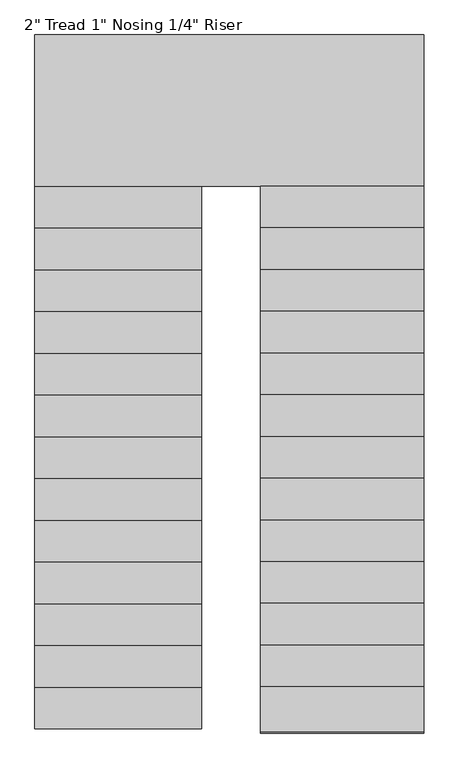
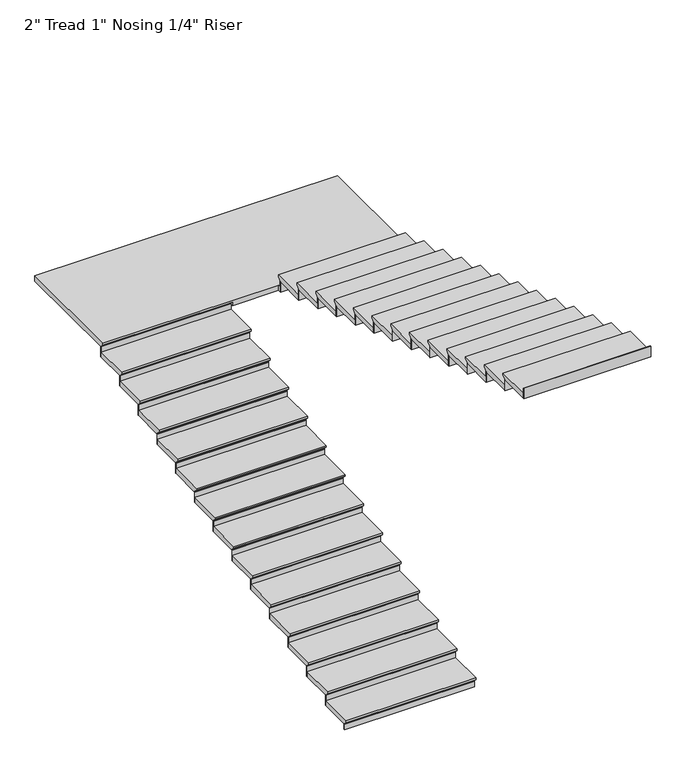
"""IFC4 building model written with IfcOpenShell, lengths in millimetres: stair flight geometry."""

from ifc_helpers import new_model, si_unit, origin, place, context, project, spatial, faceted_brep, source, transform, mapped, element, save


def stair_flight_d167e677(model_context):
    return source(origin(), model_context, "Body", "Brep", [
        faceted_brep([(-629.5987998, 2564.5067329, 6485.1642857), (-629.5987998, 2564.5067329, 6504.2142857), (-1848.7987998, 2564.5067329, 6504.2142857), (-1848.7987998, 2564.5067329, 6485.1642857), (-629.5987998, 2589.9067329, 6459.7642857), (-1848.7987998, 2589.9067329, 6459.7642857), (-629.5987998, 2894.7067329, 6504.2142857), (-1848.7987998, 2894.7067329, 6504.2142857), (-1848.7987998, 2589.9067329, 6453.4142857), (-1848.7987998, 2894.7067329, 6453.4142857), (-629.5987998, 2894.7067329, 6453.4142857), (-629.5987998, 2589.9067329, 6453.4142857)], [[[0, 1, 2, 3]], [[4, 0, 3, 5]], [[2, 1, 6, 7]], [[8, 9, 10, 11]], [[2, 7, 9, 8, 5, 3]], [[8, 11, 4, 5]], [[6, 1, 0, 4, 11, 10]], [[7, 6, 10, 9]]]),
        faceted_brep([(-629.5987998, 2589.9067329, 6453.4142857), (-629.5987998, 2589.9067329, 6400.8), (-629.5987998, 2596.2567329, 6400.8), (-629.5987998, 2596.2567329, 6453.4142857), (-1848.7987998, 2589.9067329, 6453.4142857), (-1848.7987998, 2596.2567329, 6453.4142857), (-1848.7987998, 2596.2567329, 6400.8), (-1848.7987998, 2589.9067329, 6400.8)], [[[0, 1, 2, 3]], [[4, 5, 6, 7]], [[1, 0, 4, 7]], [[2, 1, 7, 6]], [[3, 2, 6, 5]], [[0, 3, 5, 4]]]),
        faceted_brep([(-629.5987998, 2894.7067329, 6556.8285714), (-629.5987998, 2894.7067329, 6453.4142857), (-629.5987998, 2901.0567329, 6453.4142857), (-629.5987998, 2901.0567329, 6556.8285714), (-1848.7987998, 2894.7067329, 6556.8285714), (-1848.7987998, 2901.0567329, 6556.8285714), (-1848.7987998, 2901.0567329, 6453.4142857), (-1848.7987998, 2894.7067329, 6453.4142857)], [[[0, 1, 2, 3]], [[4, 5, 6, 7]], [[1, 0, 4, 7]], [[2, 1, 7, 6]], [[3, 2, 6, 5]], [[0, 3, 5, 4]]]),
        faceted_brep([(-1848.7987998, 2869.3067329, 6607.6285714), (-629.5987998, 2869.3067329, 6607.6285714), (-629.5987998, 3199.5067329, 6607.6285714), (-1848.7987998, 3199.5067329, 6607.6285714), (-1848.7987998, 2894.7067329, 6556.8285714), (-1848.7987998, 3199.5067329, 6556.8285714), (-629.5987998, 3199.5067329, 6556.8285714), (-629.5987998, 2894.7067329, 6556.8285714), (-1848.7987998, 2894.7067329, 6563.1785714), (-1848.7987998, 2869.3067329, 6588.5785714), (-629.5987998, 2894.7067329, 6563.1785714), (-629.5987998, 2869.3067329, 6588.5785714)], [[[0, 1, 2, 3]], [[4, 5, 6, 7]], [[0, 3, 5, 4, 8, 9]], [[4, 7, 10, 8]], [[2, 1, 11, 10, 7, 6]], [[3, 2, 6, 5]], [[11, 1, 0, 9]], [[10, 11, 9, 8]]]),
        faceted_brep([(-629.5987998, 3199.5067329, 6660.2428571), (-629.5987998, 3199.5067329, 6556.8285714), (-629.5987998, 3205.8567329, 6556.8285714), (-629.5987998, 3205.8567329, 6660.2428571), (-1848.7987998, 3199.5067329, 6660.2428571), (-1848.7987998, 3205.8567329, 6660.2428571), (-1848.7987998, 3205.8567329, 6556.8285714), (-1848.7987998, 3199.5067329, 6556.8285714)], [[[0, 1, 2, 3]], [[4, 5, 6, 7]], [[1, 0, 4, 7]], [[2, 1, 7, 6]], [[3, 2, 6, 5]], [[0, 3, 5, 4]]]),
        faceted_brep([(-1848.7987998, 3174.1067329, 6711.0428571), (-629.5987998, 3174.1067329, 6711.0428571), (-629.5987998, 3504.3067329, 6711.0428571), (-1848.7987998, 3504.3067329, 6711.0428571), (-1848.7987998, 3199.5067329, 6660.2428571), (-1848.7987998, 3504.3067329, 6660.2428571), (-629.5987998, 3504.3067329, 6660.2428571), (-629.5987998, 3199.5067329, 6660.2428571), (-1848.7987998, 3199.5067329, 6666.5928571), (-1848.7987998, 3174.1067329, 6691.9928571), (-629.5987998, 3199.5067329, 6666.5928571), (-629.5987998, 3174.1067329, 6691.9928571)], [[[0, 1, 2, 3]], [[4, 5, 6, 7]], [[0, 3, 5, 4, 8, 9]], [[4, 7, 10, 8]], [[2, 1, 11, 10, 7, 6]], [[3, 2, 6, 5]], [[11, 1, 0, 9]], [[10, 11, 9, 8]]]),
        faceted_brep([(-629.5987998, 3504.3067329, 6763.6571429), (-629.5987998, 3504.3067329, 6660.2428571), (-629.5987998, 3510.6567329, 6660.2428571), (-629.5987998, 3510.6567329, 6763.6571429), (-1848.7987998, 3504.3067329, 6763.6571429), (-1848.7987998, 3510.6567329, 6763.6571429), (-1848.7987998, 3510.6567329, 6660.2428571), (-1848.7987998, 3504.3067329, 6660.2428571)], [[[0, 1, 2, 3]], [[4, 5, 6, 7]], [[1, 0, 4, 7]], [[2, 1, 7, 6]], [[3, 2, 6, 5]], [[0, 3, 5, 4]]]),
        faceted_brep([(-1848.7987998, 3478.9067329, 6814.4571429), (-629.5987998, 3478.9067329, 6814.4571429), (-629.5987998, 3809.1067329, 6814.4571429), (-1848.7987998, 3809.1067329, 6814.4571429), (-1848.7987998, 3504.3067329, 6763.6571429), (-1848.7987998, 3809.1067329, 6763.6571429), (-629.5987998, 3809.1067329, 6763.6571429), (-629.5987998, 3504.3067329, 6763.6571429), (-1848.7987998, 3504.3067329, 6770.0071429), (-1848.7987998, 3478.9067329, 6795.4071429), (-629.5987998, 3504.3067329, 6770.0071429), (-629.5987998, 3478.9067329, 6795.4071429)], [[[0, 1, 2, 3]], [[4, 5, 6, 7]], [[0, 3, 5, 4, 8, 9]], [[4, 7, 10, 8]], [[2, 1, 11, 10, 7, 6]], [[3, 2, 6, 5]], [[11, 1, 0, 9]], [[10, 11, 9, 8]]]),
        faceted_brep([(-629.5987998, 3809.1067329, 6867.0714286), (-629.5987998, 3809.1067329, 6763.6571429), (-629.5987998, 3815.4567329, 6763.6571429), (-629.5987998, 3815.4567329, 6867.0714286), (-1848.7987998, 3809.1067329, 6867.0714286), (-1848.7987998, 3815.4567329, 6867.0714286), (-1848.7987998, 3815.4567329, 6763.6571429), (-1848.7987998, 3809.1067329, 6763.6571429)], [[[0, 1, 2, 3]], [[4, 5, 6, 7]], [[1, 0, 4, 7]], [[2, 1, 7, 6]], [[3, 2, 6, 5]], [[0, 3, 5, 4]]]),
        faceted_brep([(-1848.7987998, 3783.7067329, 6917.8714286), (-629.5987998, 3783.7067329, 6917.8714286), (-629.5987998, 4113.9067329, 6917.8714286), (-1848.7987998, 4113.9067329, 6917.8714286), (-1848.7987998, 3809.1067329, 6867.0714286), (-1848.7987998, 4113.9067329, 6867.0714286), (-629.5987998, 4113.9067329, 6867.0714286), (-629.5987998, 3809.1067329, 6867.0714286), (-1848.7987998, 3809.1067329, 6873.4214286), (-1848.7987998, 3783.7067329, 6898.8214286), (-629.5987998, 3809.1067329, 6873.4214286), (-629.5987998, 3783.7067329, 6898.8214286)], [[[0, 1, 2, 3]], [[4, 5, 6, 7]], [[0, 3, 5, 4, 8, 9]], [[4, 7, 10, 8]], [[2, 1, 11, 10, 7, 6]], [[3, 2, 6, 5]], [[11, 1, 0, 9]], [[10, 11, 9, 8]]]),
        faceted_brep([(-629.5987998, 4113.9067329, 6970.4857143), (-629.5987998, 4113.9067329, 6867.0714286), (-629.5987998, 4120.2567329, 6867.0714286), (-629.5987998, 4120.2567329, 6970.4857143), (-1848.7987998, 4113.9067329, 6970.4857143), (-1848.7987998, 4120.2567329, 6970.4857143), (-1848.7987998, 4120.2567329, 6867.0714286), (-1848.7987998, 4113.9067329, 6867.0714286)], [[[0, 1, 2, 3]], [[4, 5, 6, 7]], [[1, 0, 4, 7]], [[2, 1, 7, 6]], [[3, 2, 6, 5]], [[0, 3, 5, 4]]]),
        faceted_brep([(-1848.7987998, 4088.5067329, 7021.2857143), (-629.5987998, 4088.5067329, 7021.2857143), (-629.5987998, 4418.7067329, 7021.2857143), (-1848.7987998, 4418.7067329, 7021.2857143), (-1848.7987998, 4113.9067329, 6970.4857143), (-1848.7987998, 4418.7067329, 6970.4857143), (-629.5987998, 4418.7067329, 6970.4857143), (-629.5987998, 4113.9067329, 6970.4857143), (-1848.7987998, 4113.9067329, 6976.8357143), (-1848.7987998, 4088.5067329, 7002.2357143), (-629.5987998, 4113.9067329, 6976.8357143), (-629.5987998, 4088.5067329, 7002.2357143)], [[[0, 1, 2, 3]], [[4, 5, 6, 7]], [[0, 3, 5, 4, 8, 9]], [[4, 7, 10, 8]], [[2, 1, 11, 10, 7, 6]], [[3, 2, 6, 5]], [[11, 1, 0, 9]], [[10, 11, 9, 8]]]),
        faceted_brep([(-629.5987998, 4418.7067329, 7073.9), (-629.5987998, 4418.7067329, 6970.4857143), (-629.5987998, 4425.0567329, 6970.4857143), (-629.5987998, 4425.0567329, 7073.9), (-1848.7987998, 4418.7067329, 7073.9), (-1848.7987998, 4425.0567329, 7073.9), (-1848.7987998, 4425.0567329, 6970.4857143), (-1848.7987998, 4418.7067329, 6970.4857143)], [[[0, 1, 2, 3]], [[4, 5, 6, 7]], [[1, 0, 4, 7]], [[2, 1, 7, 6]], [[3, 2, 6, 5]], [[0, 3, 5, 4]]]),
        faceted_brep([(-1848.7987998, 4393.3067329, 7124.7), (-629.5987998, 4393.3067329, 7124.7), (-629.5987998, 4723.5067329, 7124.7), (-1848.7987998, 4723.5067329, 7124.7), (-1848.7987998, 4418.7067329, 7073.9), (-1848.7987998, 4723.5067329, 7073.9), (-629.5987998, 4723.5067329, 7073.9), (-629.5987998, 4418.7067329, 7073.9), (-1848.7987998, 4418.7067329, 7080.25), (-1848.7987998, 4393.3067329, 7105.65), (-629.5987998, 4418.7067329, 7080.25), (-629.5987998, 4393.3067329, 7105.65)], [[[0, 1, 2, 3]], [[4, 5, 6, 7]], [[0, 3, 5, 4, 8, 9]], [[4, 7, 10, 8]], [[2, 1, 11, 10, 7, 6]], [[3, 2, 6, 5]], [[11, 1, 0, 9]], [[10, 11, 9, 8]]]),
        faceted_brep([(-629.5987998, 4723.5067329, 7177.3142857), (-629.5987998, 4723.5067329, 7073.9), (-629.5987998, 4729.8567329, 7073.9), (-629.5987998, 4729.8567329, 7177.3142857), (-1848.7987998, 4723.5067329, 7177.3142857), (-1848.7987998, 4729.8567329, 7177.3142857), (-1848.7987998, 4729.8567329, 7073.9), (-1848.7987998, 4723.5067329, 7073.9)], [[[0, 1, 2, 3]], [[4, 5, 6, 7]], [[1, 0, 4, 7]], [[2, 1, 7, 6]], [[3, 2, 6, 5]], [[0, 3, 5, 4]]]),
        faceted_brep([(-1848.7987998, 4698.1067329, 7228.1142857), (-629.5987998, 4698.1067329, 7228.1142857), (-629.5987998, 5028.3067329, 7228.1142857), (-1848.7987998, 5028.3067329, 7228.1142857), (-1848.7987998, 4723.5067329, 7177.3142857), (-1848.7987998, 5028.3067329, 7177.3142857), (-629.5987998, 5028.3067329, 7177.3142857), (-629.5987998, 4723.5067329, 7177.3142857), (-1848.7987998, 4723.5067329, 7183.6642857), (-1848.7987998, 4698.1067329, 7209.0642857), (-629.5987998, 4723.5067329, 7183.6642857), (-629.5987998, 4698.1067329, 7209.0642857)], [[[0, 1, 2, 3]], [[4, 5, 6, 7]], [[0, 3, 5, 4, 8, 9]], [[4, 7, 10, 8]], [[2, 1, 11, 10, 7, 6]], [[3, 2, 6, 5]], [[11, 1, 0, 9]], [[10, 11, 9, 8]]]),
        faceted_brep([(-629.5987998, 5028.3067329, 7280.7285714), (-629.5987998, 5028.3067329, 7177.3142857), (-629.5987998, 5034.6567329, 7177.3142857), (-629.5987998, 5034.6567329, 7280.7285714), (-1848.7987998, 5028.3067329, 7280.7285714), (-1848.7987998, 5034.6567329, 7280.7285714), (-1848.7987998, 5034.6567329, 7177.3142857), (-1848.7987998, 5028.3067329, 7177.3142857)], [[[0, 1, 2, 3]], [[4, 5, 6, 7]], [[1, 0, 4, 7]], [[2, 1, 7, 6]], [[3, 2, 6, 5]], [[0, 3, 5, 4]]]),
        faceted_brep([(-1848.7987998, 5002.9067329, 7331.5285714), (-629.5987998, 5002.9067329, 7331.5285714), (-629.5987998, 5333.1067329, 7331.5285714), (-1848.7987998, 5333.1067329, 7331.5285714), (-1848.7987998, 5028.3067329, 7280.7285714), (-1848.7987998, 5333.1067329, 7280.7285714), (-629.5987998, 5333.1067329, 7280.7285714), (-629.5987998, 5028.3067329, 7280.7285714), (-1848.7987998, 5028.3067329, 7287.0785714), (-1848.7987998, 5002.9067329, 7312.4785714), (-629.5987998, 5028.3067329, 7287.0785714), (-629.5987998, 5002.9067329, 7312.4785714)], [[[0, 1, 2, 3]], [[4, 5, 6, 7]], [[0, 3, 5, 4, 8, 9]], [[4, 7, 10, 8]], [[2, 1, 11, 10, 7, 6]], [[3, 2, 6, 5]], [[11, 1, 0, 9]], [[10, 11, 9, 8]]]),
        faceted_brep([(-629.5987998, 5333.1067329, 7384.1428571), (-629.5987998, 5333.1067329, 7280.7285714), (-629.5987998, 5339.4567329, 7280.7285714), (-629.5987998, 5339.4567329, 7384.1428571), (-1848.7987998, 5333.1067329, 7384.1428571), (-1848.7987998, 5339.4567329, 7384.1428571), (-1848.7987998, 5339.4567329, 7280.7285714), (-1848.7987998, 5333.1067329, 7280.7285714)], [[[0, 1, 2, 3]], [[4, 5, 6, 7]], [[1, 0, 4, 7]], [[2, 1, 7, 6]], [[3, 2, 6, 5]], [[0, 3, 5, 4]]]),
        faceted_brep([(-1848.7987998, 5307.7067329, 7434.9428571), (-629.5987998, 5307.7067329, 7434.9428571), (-629.5987998, 5637.9067329, 7434.9428571), (-1848.7987998, 5637.9067329, 7434.9428571), (-1848.7987998, 5333.1067329, 7384.1428571), (-1848.7987998, 5637.9067329, 7384.1428571), (-629.5987998, 5637.9067329, 7384.1428571), (-629.5987998, 5333.1067329, 7384.1428571), (-1848.7987998, 5333.1067329, 7390.4928571), (-1848.7987998, 5307.7067329, 7415.8928571), (-629.5987998, 5333.1067329, 7390.4928571), (-629.5987998, 5307.7067329, 7415.8928571)], [[[0, 1, 2, 3]], [[4, 5, 6, 7]], [[0, 3, 5, 4, 8, 9]], [[4, 7, 10, 8]], [[2, 1, 11, 10, 7, 6]], [[3, 2, 6, 5]], [[11, 1, 0, 9]], [[10, 11, 9, 8]]]),
        faceted_brep([(-629.5987998, 5637.9067329, 7487.5571429), (-629.5987998, 5637.9067329, 7384.1428571), (-629.5987998, 5644.2567329, 7384.1428571), (-629.5987998, 5644.2567329, 7487.5571429), (-1848.7987998, 5637.9067329, 7487.5571429), (-1848.7987998, 5644.2567329, 7487.5571429), (-1848.7987998, 5644.2567329, 7384.1428571), (-1848.7987998, 5637.9067329, 7384.1428571)], [[[0, 1, 2, 3]], [[4, 5, 6, 7]], [[1, 0, 4, 7]], [[2, 1, 7, 6]], [[3, 2, 6, 5]], [[0, 3, 5, 4]]]),
        faceted_brep([(-1848.7987998, 5612.5067329, 7538.3571429), (-629.5987998, 5612.5067329, 7538.3571429), (-629.5987998, 5942.7067329, 7538.3571429), (-1848.7987998, 5942.7067329, 7538.3571429), (-1848.7987998, 5637.9067329, 7487.5571429), (-1848.7987998, 5942.7067329, 7487.5571429), (-629.5987998, 5942.7067329, 7487.5571429), (-629.5987998, 5637.9067329, 7487.5571429), (-1848.7987998, 5637.9067329, 7493.9071429), (-1848.7987998, 5612.5067329, 7519.3071429), (-629.5987998, 5637.9067329, 7493.9071429), (-629.5987998, 5612.5067329, 7519.3071429)], [[[0, 1, 2, 3]], [[4, 5, 6, 7]], [[0, 3, 5, 4, 8, 9]], [[4, 7, 10, 8]], [[2, 1, 11, 10, 7, 6]], [[3, 2, 6, 5]], [[11, 1, 0, 9]], [[10, 11, 9, 8]]]),
        faceted_brep([(-629.5987998, 5942.7067329, 7590.9714286), (-629.5987998, 5942.7067329, 7487.5571429), (-629.5987998, 5949.0567329, 7487.5571429), (-629.5987998, 5949.0567329, 7590.9714286), (-1848.7987998, 5942.7067329, 7590.9714286), (-1848.7987998, 5949.0567329, 7590.9714286), (-1848.7987998, 5949.0567329, 7487.5571429), (-1848.7987998, 5942.7067329, 7487.5571429)], [[[0, 1, 2, 3]], [[4, 5, 6, 7]], [[1, 0, 4, 7]], [[2, 1, 7, 6]], [[3, 2, 6, 5]], [[0, 3, 5, 4]]]),
        faceted_brep([(-1848.7987998, 5917.3067329, 7641.7714286), (-629.5987998, 5917.3067329, 7641.7714286), (-629.5987998, 6247.5067329, 7641.7714286), (-1848.7987998, 6247.5067329, 7641.7714286), (-1848.7987998, 5942.7067329, 7590.9714286), (-1848.7987998, 6247.5067329, 7590.9714286), (-629.5987998, 6247.5067329, 7590.9714286), (-629.5987998, 5942.7067329, 7590.9714286), (-1848.7987998, 5942.7067329, 7597.3214286), (-1848.7987998, 5917.3067329, 7622.7214286), (-629.5987998, 5942.7067329, 7597.3214286), (-629.5987998, 5917.3067329, 7622.7214286)], [[[0, 1, 2, 3]], [[4, 5, 6, 7]], [[0, 3, 5, 4, 8, 9]], [[4, 7, 10, 8]], [[2, 1, 11, 10, 7, 6]], [[3, 2, 6, 5]], [[11, 1, 0, 9]], [[10, 11, 9, 8]]]),
        faceted_brep([(-629.5987998, 6247.5067329, 7694.3857143), (-629.5987998, 6247.5067329, 7590.9714286), (-629.5987998, 6253.8567329, 7590.9714286), (-629.5987998, 6253.8567329, 7694.3857143), (-1848.7987998, 6247.5067329, 7694.3857143), (-1848.7987998, 6253.8567329, 7694.3857143), (-1848.7987998, 6253.8567329, 7590.9714286), (-1848.7987998, 6247.5067329, 7590.9714286)], [[[0, 1, 2, 3]], [[4, 5, 6, 7]], [[1, 0, 4, 7]], [[2, 1, 7, 6]], [[3, 2, 6, 5]], [[0, 3, 5, 4]]]),
        faceted_brep([(-1848.7987998, 6222.1067329, 7745.1857143), (-629.5987998, 6222.1067329, 7745.1857143), (-629.5987998, 6552.3067329, 7745.1857143), (-1848.7987998, 6552.3067329, 7745.1857143), (-1848.7987998, 6247.5067329, 7694.3857143), (-1848.7987998, 6552.3067329, 7694.3857143), (-629.5987998, 6552.3067329, 7694.3857143), (-629.5987998, 6247.5067329, 7694.3857143), (-1848.7987998, 6247.5067329, 7700.7357143), (-1848.7987998, 6222.1067329, 7726.1357143), (-629.5987998, 6247.5067329, 7700.7357143), (-629.5987998, 6222.1067329, 7726.1357143)], [[[0, 1, 2, 3]], [[4, 5, 6, 7]], [[0, 3, 5, 4, 8, 9]], [[4, 7, 10, 8]], [[2, 1, 11, 10, 7, 6]], [[3, 2, 6, 5]], [[11, 1, 0, 9]], [[10, 11, 9, 8]]]),
        faceted_brep([(-629.5987998, 6552.3067329, 7797.8), (-629.5987998, 6552.3067329, 7694.3857143), (-629.5987998, 6558.6567329, 7694.3857143), (-629.5987998, 6558.6567329, 7797.8), (-1848.7987998, 6552.3067329, 7797.8), (-1848.7987998, 6558.6567329, 7797.8), (-1848.7987998, 6558.6567329, 7694.3857143), (-1848.7987998, 6552.3067329, 7694.3857143)], [[[0, 1, 2, 3]], [[4, 5, 6, 7]], [[1, 0, 4, 7]], [[2, 1, 7, 6]], [[3, 2, 6, 5]], [[0, 3, 5, 4]]]),
        faceted_brep([(996.0012002, 6501.5067329, 7848.6), (996.0012002, 7631.8067329, 7848.6), (-1848.7987998, 7631.8067329, 7848.6), (-1848.7987998, 6526.9067329, 7848.6), (-197.7987915, 6526.9067329, 7848.6), (-197.7987915, 6501.5067329, 7848.6), (996.0012002, 7631.8067329, 7797.8), (996.0012002, 6501.5067329, 7797.8), (-197.7987915, 6501.5067329, 7797.8), (-197.7987915, 6526.9067329, 7797.8), (-629.5987998, 6526.9067329, 7797.8), (-629.5987998, 6552.3067329, 7797.8), (-1848.7987998, 6552.3067329, 7797.8), (-1848.7987998, 7631.8067329, 7797.8), (-629.5987998, 6552.3067329, 7804.15), (-1848.7987998, 6552.3067329, 7804.15), (-1848.7987998, 6526.9067329, 7829.55), (-629.5987998, 6526.9067329, 7829.55)], [[[0, 1, 2, 3, 4, 5]], [[6, 7, 8, 9, 10, 11, 12, 13]], [[1, 0, 7, 6]], [[2, 1, 6, 13]], [[12, 11, 14, 15]], [[4, 3, 16, 17, 10, 9]], [[5, 4, 9, 8]], [[0, 5, 8, 7]], [[16, 15, 14, 17]], [[3, 2, 13, 12, 15, 16]], [[11, 10, 17, 14]]]),
        faceted_brep([(-197.7987915, 6501.5067329, 7901.2142857), (-197.7987915, 6501.5067329, 7797.8), (-197.7987915, 6495.1567329, 7797.8), (-197.7987915, 6495.1567329, 7901.2142857), (996.0012002, 6501.5067329, 7901.2142857), (996.0012002, 6495.1567329, 7901.2142857), (996.0012002, 6495.1567329, 7797.8), (996.0012002, 6501.5067329, 7797.8)], [[[0, 1, 2, 3]], [[4, 5, 6, 7]], [[1, 0, 4, 7]], [[2, 1, 7, 6]], [[3, 2, 6, 5]], [[0, 3, 5, 4]]]),
        faceted_brep([(996.0012002, 6526.9067329, 7952.0142857), (-197.7987915, 6526.9067329, 7952.0142857), (-197.7987915, 6196.7067329, 7952.0142857), (996.0012002, 6196.7067329, 7952.0142857), (996.0012002, 6501.5067329, 7901.2142857), (996.0012002, 6196.7067329, 7901.2142857), (-197.7987915, 6196.7067329, 7901.2142857), (-197.7987915, 6501.5067329, 7901.2142857), (996.0012002, 6501.5067329, 7907.5642857), (996.0012002, 6526.9067329, 7932.9642857), (-197.7987915, 6501.5067329, 7907.5642857), (-197.7987915, 6526.9067329, 7932.9642857)], [[[0, 1, 2, 3]], [[4, 5, 6, 7]], [[0, 3, 5, 4, 8, 9]], [[4, 7, 10, 8]], [[2, 1, 11, 10, 7, 6]], [[3, 2, 6, 5]], [[11, 1, 0, 9]], [[10, 11, 9, 8]]]),
        faceted_brep([(-197.7987915, 6196.7067329, 8004.6285714), (-197.7987915, 6196.7067329, 7901.2142857), (-197.7987915, 6190.3567329, 7901.2142857), (-197.7987915, 6190.3567329, 8004.6285714), (996.0012002, 6196.7067329, 8004.6285714), (996.0012002, 6190.3567329, 8004.6285714), (996.0012002, 6190.3567329, 7901.2142857), (996.0012002, 6196.7067329, 7901.2142857)], [[[0, 1, 2, 3]], [[4, 5, 6, 7]], [[1, 0, 4, 7]], [[2, 1, 7, 6]], [[3, 2, 6, 5]], [[0, 3, 5, 4]]]),
        faceted_brep([(996.0012002, 6222.1067329, 8055.4285714), (-197.7987915, 6222.1067329, 8055.4285714), (-197.7987915, 5891.9067329, 8055.4285714), (996.0012002, 5891.9067329, 8055.4285714), (996.0012002, 6196.7067329, 8004.6285714), (996.0012002, 5891.9067329, 8004.6285714), (-197.7987915, 5891.9067329, 8004.6285714), (-197.7987915, 6196.7067329, 8004.6285714), (996.0012002, 6196.7067329, 8010.9785714), (996.0012002, 6222.1067329, 8036.3785714), (-197.7987915, 6196.7067329, 8010.9785714), (-197.7987915, 6222.1067329, 8036.3785714)], [[[0, 1, 2, 3]], [[4, 5, 6, 7]], [[0, 3, 5, 4, 8, 9]], [[4, 7, 10, 8]], [[2, 1, 11, 10, 7, 6]], [[3, 2, 6, 5]], [[11, 1, 0, 9]], [[10, 11, 9, 8]]]),
        faceted_brep([(-197.7987915, 5891.9067329, 8108.0428571), (-197.7987915, 5891.9067329, 8004.6285714), (-197.7987915, 5885.5567329, 8004.6285714), (-197.7987915, 5885.5567329, 8108.0428571), (996.0012002, 5891.9067329, 8108.0428571), (996.0012002, 5885.5567329, 8108.0428571), (996.0012002, 5885.5567329, 8004.6285714), (996.0012002, 5891.9067329, 8004.6285714)], [[[0, 1, 2, 3]], [[4, 5, 6, 7]], [[1, 0, 4, 7]], [[2, 1, 7, 6]], [[3, 2, 6, 5]], [[0, 3, 5, 4]]]),
        faceted_brep([(996.0012002, 5917.3067329, 8158.8428571), (-197.7987915, 5917.3067329, 8158.8428571), (-197.7987915, 5587.1067329, 8158.8428571), (996.0012002, 5587.1067329, 8158.8428571), (996.0012002, 5891.9067329, 8108.0428571), (996.0012002, 5587.1067329, 8108.0428571), (-197.7987915, 5587.1067329, 8108.0428571), (-197.7987915, 5891.9067329, 8108.0428571), (996.0012002, 5891.9067329, 8114.3928571), (996.0012002, 5917.3067329, 8139.7928571), (-197.7987915, 5891.9067329, 8114.3928571), (-197.7987915, 5917.3067329, 8139.7928571)], [[[0, 1, 2, 3]], [[4, 5, 6, 7]], [[0, 3, 5, 4, 8, 9]], [[4, 7, 10, 8]], [[2, 1, 11, 10, 7, 6]], [[3, 2, 6, 5]], [[11, 1, 0, 9]], [[10, 11, 9, 8]]]),
        faceted_brep([(-197.7987915, 5587.1067329, 8211.4571429), (-197.7987915, 5587.1067329, 8108.0428571), (-197.7987915, 5580.7567329, 8108.0428571), (-197.7987915, 5580.7567329, 8211.4571429), (996.0012002, 5587.1067329, 8211.4571429), (996.0012002, 5580.7567329, 8211.4571429), (996.0012002, 5580.7567329, 8108.0428571), (996.0012002, 5587.1067329, 8108.0428571)], [[[0, 1, 2, 3]], [[4, 5, 6, 7]], [[1, 0, 4, 7]], [[2, 1, 7, 6]], [[3, 2, 6, 5]], [[0, 3, 5, 4]]]),
        faceted_brep([(996.0012002, 5612.5067329, 8262.2571429), (-197.7987915, 5612.5067329, 8262.2571429), (-197.7987915, 5282.3067329, 8262.2571429), (996.0012002, 5282.3067329, 8262.2571429), (996.0012002, 5587.1067329, 8211.4571429), (996.0012002, 5282.3067329, 8211.4571429), (-197.7987915, 5282.3067329, 8211.4571429), (-197.7987915, 5587.1067329, 8211.4571429), (996.0012002, 5587.1067329, 8217.8071429), (996.0012002, 5612.5067329, 8243.2071429), (-197.7987915, 5587.1067329, 8217.8071429), (-197.7987915, 5612.5067329, 8243.2071429)], [[[0, 1, 2, 3]], [[4, 5, 6, 7]], [[0, 3, 5, 4, 8, 9]], [[4, 7, 10, 8]], [[2, 1, 11, 10, 7, 6]], [[3, 2, 6, 5]], [[11, 1, 0, 9]], [[10, 11, 9, 8]]]),
        faceted_brep([(-197.7987915, 5282.3067329, 8314.8714286), (-197.7987915, 5282.3067329, 8211.4571429), (-197.7987915, 5275.9567329, 8211.4571429), (-197.7987915, 5275.9567329, 8314.8714286), (996.0012002, 5282.3067329, 8314.8714286), (996.0012002, 5275.9567329, 8314.8714286), (996.0012002, 5275.9567329, 8211.4571429), (996.0012002, 5282.3067329, 8211.4571429)], [[[0, 1, 2, 3]], [[4, 5, 6, 7]], [[1, 0, 4, 7]], [[2, 1, 7, 6]], [[3, 2, 6, 5]], [[0, 3, 5, 4]]]),
        faceted_brep([(996.0012002, 5307.7067329, 8365.6714286), (-197.7987915, 5307.7067329, 8365.6714286), (-197.7987915, 4977.5067329, 8365.6714286), (996.0012002, 4977.5067329, 8365.6714286), (996.0012002, 5282.3067329, 8314.8714286), (996.0012002, 4977.5067329, 8314.8714286), (-197.7987915, 4977.5067329, 8314.8714286), (-197.7987915, 5282.3067329, 8314.8714286), (996.0012002, 5282.3067329, 8321.2214286), (996.0012002, 5307.7067329, 8346.6214286), (-197.7987915, 5282.3067329, 8321.2214286), (-197.7987915, 5307.7067329, 8346.6214286)], [[[0, 1, 2, 3]], [[4, 5, 6, 7]], [[0, 3, 5, 4, 8, 9]], [[4, 7, 10, 8]], [[2, 1, 11, 10, 7, 6]], [[3, 2, 6, 5]], [[11, 1, 0, 9]], [[10, 11, 9, 8]]]),
        faceted_brep([(-197.7987915, 4977.5067329, 8418.2857143), (-197.7987915, 4977.5067329, 8314.8714286), (-197.7987915, 4971.1567329, 8314.8714286), (-197.7987915, 4971.1567329, 8418.2857143), (996.0012002, 4977.5067329, 8418.2857143), (996.0012002, 4971.1567329, 8418.2857143), (996.0012002, 4971.1567329, 8314.8714286), (996.0012002, 4977.5067329, 8314.8714286)], [[[0, 1, 2, 3]], [[4, 5, 6, 7]], [[1, 0, 4, 7]], [[2, 1, 7, 6]], [[3, 2, 6, 5]], [[0, 3, 5, 4]]]),
        faceted_brep([(996.0012002, 5002.9067329, 8469.0857143), (-197.7987915, 5002.9067329, 8469.0857143), (-197.7987915, 4672.7067329, 8469.0857143), (996.0012002, 4672.7067329, 8469.0857143), (996.0012002, 4977.5067329, 8418.2857143), (996.0012002, 4672.7067329, 8418.2857143), (-197.7987915, 4672.7067329, 8418.2857143), (-197.7987915, 4977.5067329, 8418.2857143), (996.0012002, 4977.5067329, 8424.6357143), (996.0012002, 5002.9067329, 8450.0357143), (-197.7987915, 4977.5067329, 8424.6357143), (-197.7987915, 5002.9067329, 8450.0357143)], [[[0, 1, 2, 3]], [[4, 5, 6, 7]], [[0, 3, 5, 4, 8, 9]], [[4, 7, 10, 8]], [[2, 1, 11, 10, 7, 6]], [[3, 2, 6, 5]], [[11, 1, 0, 9]], [[10, 11, 9, 8]]]),
        faceted_brep([(-197.7987915, 4672.7067329, 8521.7), (-197.7987915, 4672.7067329, 8418.2857143), (-197.7987915, 4666.3567329, 8418.2857143), (-197.7987915, 4666.3567329, 8521.7), (996.0012002, 4672.7067329, 8521.7), (996.0012002, 4666.3567329, 8521.7), (996.0012002, 4666.3567329, 8418.2857143), (996.0012002, 4672.7067329, 8418.2857143)], [[[0, 1, 2, 3]], [[4, 5, 6, 7]], [[1, 0, 4, 7]], [[2, 1, 7, 6]], [[3, 2, 6, 5]], [[0, 3, 5, 4]]]),
        faceted_brep([(996.0012002, 4698.1067329, 8572.5), (-197.7987915, 4698.1067329, 8572.5), (-197.7987915, 4367.9067329, 8572.5), (996.0012002, 4367.9067329, 8572.5), (996.0012002, 4672.7067329, 8521.7), (996.0012002, 4367.9067329, 8521.7), (-197.7987915, 4367.9067329, 8521.7), (-197.7987915, 4672.7067329, 8521.7), (996.0012002, 4672.7067329, 8528.05), (996.0012002, 4698.1067329, 8553.45), (-197.7987915, 4672.7067329, 8528.05), (-197.7987915, 4698.1067329, 8553.45)], [[[0, 1, 2, 3]], [[4, 5, 6, 7]], [[0, 3, 5, 4, 8, 9]], [[4, 7, 10, 8]], [[2, 1, 11, 10, 7, 6]], [[3, 2, 6, 5]], [[11, 1, 0, 9]], [[10, 11, 9, 8]]]),
        faceted_brep([(-197.7987915, 4367.9067329, 8625.1142857), (-197.7987915, 4367.9067329, 8521.7), (-197.7987915, 4361.5567329, 8521.7), (-197.7987915, 4361.5567329, 8625.1142857), (996.0012002, 4367.9067329, 8625.1142857), (996.0012002, 4361.5567329, 8625.1142857), (996.0012002, 4361.5567329, 8521.7), (996.0012002, 4367.9067329, 8521.7)], [[[0, 1, 2, 3]], [[4, 5, 6, 7]], [[1, 0, 4, 7]], [[2, 1, 7, 6]], [[3, 2, 6, 5]], [[0, 3, 5, 4]]]),
        faceted_brep([(996.0012002, 4393.3067329, 8675.9142857), (-197.7987915, 4393.3067329, 8675.9142857), (-197.7987915, 4063.1067329, 8675.9142857), (996.0012002, 4063.1067329, 8675.9142857), (996.0012002, 4367.9067329, 8625.1142857), (996.0012002, 4063.1067329, 8625.1142857), (-197.7987915, 4063.1067329, 8625.1142857), (-197.7987915, 4367.9067329, 8625.1142857), (996.0012002, 4367.9067329, 8631.4642857), (996.0012002, 4393.3067329, 8656.8642857), (-197.7987915, 4367.9067329, 8631.4642857), (-197.7987915, 4393.3067329, 8656.8642857)], [[[0, 1, 2, 3]], [[4, 5, 6, 7]], [[0, 3, 5, 4, 8, 9]], [[4, 7, 10, 8]], [[2, 1, 11, 10, 7, 6]], [[3, 2, 6, 5]], [[11, 1, 0, 9]], [[10, 11, 9, 8]]]),
        faceted_brep([(-197.7987915, 4063.1067329, 8728.5285714), (-197.7987915, 4063.1067329, 8625.1142857), (-197.7987915, 4056.7567329, 8625.1142857), (-197.7987915, 4056.7567329, 8728.5285714), (996.0012002, 4063.1067329, 8728.5285714), (996.0012002, 4056.7567329, 8728.5285714), (996.0012002, 4056.7567329, 8625.1142857), (996.0012002, 4063.1067329, 8625.1142857)], [[[0, 1, 2, 3]], [[4, 5, 6, 7]], [[1, 0, 4, 7]], [[2, 1, 7, 6]], [[3, 2, 6, 5]], [[0, 3, 5, 4]]]),
        faceted_brep([(996.0012002, 4088.5067329, 8779.3285714), (-197.7987915, 4088.5067329, 8779.3285714), (-197.7987915, 3758.3067329, 8779.3285714), (996.0012002, 3758.3067329, 8779.3285714), (996.0012002, 4063.1067329, 8728.5285714), (996.0012002, 3758.3067329, 8728.5285714), (-197.7987915, 3758.3067329, 8728.5285714), (-197.7987915, 4063.1067329, 8728.5285714), (996.0012002, 4063.1067329, 8734.8785714), (996.0012002, 4088.5067329, 8760.2785714), (-197.7987915, 4063.1067329, 8734.8785714), (-197.7987915, 4088.5067329, 8760.2785714)], [[[0, 1, 2, 3]], [[4, 5, 6, 7]], [[0, 3, 5, 4, 8, 9]], [[4, 7, 10, 8]], [[2, 1, 11, 10, 7, 6]], [[3, 2, 6, 5]], [[11, 1, 0, 9]], [[10, 11, 9, 8]]]),
        faceted_brep([(-197.7987915, 3758.3067329, 8831.9428571), (-197.7987915, 3758.3067329, 8728.5285714), (-197.7987915, 3751.9567329, 8728.5285714), (-197.7987915, 3751.9567329, 8831.9428571), (996.0012002, 3758.3067329, 8831.9428571), (996.0012002, 3751.9567329, 8831.9428571), (996.0012002, 3751.9567329, 8728.5285714), (996.0012002, 3758.3067329, 8728.5285714)], [[[0, 1, 2, 3]], [[4, 5, 6, 7]], [[1, 0, 4, 7]], [[2, 1, 7, 6]], [[3, 2, 6, 5]], [[0, 3, 5, 4]]]),
        faceted_brep([(996.0012002, 3783.7067329, 8882.7428571), (-197.7987915, 3783.7067329, 8882.7428571), (-197.7987915, 3453.5067329, 8882.7428571), (996.0012002, 3453.5067329, 8882.7428571), (996.0012002, 3758.3067329, 8831.9428571), (996.0012002, 3453.5067329, 8831.9428571), (-197.7987915, 3453.5067329, 8831.9428571), (-197.7987915, 3758.3067329, 8831.9428571), (996.0012002, 3758.3067329, 8838.2928571), (996.0012002, 3783.7067329, 8863.6928571), (-197.7987915, 3758.3067329, 8838.2928571), (-197.7987915, 3783.7067329, 8863.6928571)], [[[0, 1, 2, 3]], [[4, 5, 6, 7]], [[0, 3, 5, 4, 8, 9]], [[4, 7, 10, 8]], [[2, 1, 11, 10, 7, 6]], [[3, 2, 6, 5]], [[11, 1, 0, 9]], [[10, 11, 9, 8]]]),
        faceted_brep([(-197.7987915, 3453.5067329, 8935.3571429), (-197.7987915, 3453.5067329, 8831.9428571), (-197.7987915, 3447.1567329, 8831.9428571), (-197.7987915, 3447.1567329, 8935.3571429), (996.0012002, 3453.5067329, 8935.3571429), (996.0012002, 3447.1567329, 8935.3571429), (996.0012002, 3447.1567329, 8831.9428571), (996.0012002, 3453.5067329, 8831.9428571)], [[[0, 1, 2, 3]], [[4, 5, 6, 7]], [[1, 0, 4, 7]], [[2, 1, 7, 6]], [[3, 2, 6, 5]], [[0, 3, 5, 4]]]),
        faceted_brep([(996.0012002, 3478.9067329, 8986.1571429), (-197.7987915, 3478.9067329, 8986.1571429), (-197.7987915, 3148.7067329, 8986.1571429), (996.0012002, 3148.7067329, 8986.1571429), (996.0012002, 3453.5067329, 8935.3571429), (996.0012002, 3148.7067329, 8935.3571429), (-197.7987915, 3148.7067329, 8935.3571429), (-197.7987915, 3453.5067329, 8935.3571429), (996.0012002, 3453.5067329, 8941.7071429), (996.0012002, 3478.9067329, 8967.1071429), (-197.7987915, 3453.5067329, 8941.7071429), (-197.7987915, 3478.9067329, 8967.1071429)], [[[0, 1, 2, 3]], [[4, 5, 6, 7]], [[0, 3, 5, 4, 8, 9]], [[4, 7, 10, 8]], [[2, 1, 11, 10, 7, 6]], [[3, 2, 6, 5]], [[11, 1, 0, 9]], [[10, 11, 9, 8]]]),
        faceted_brep([(-197.7987915, 3148.7067329, 9038.7714286), (-197.7987915, 3148.7067329, 8935.3571429), (-197.7987915, 3142.3567329, 8935.3571429), (-197.7987915, 3142.3567329, 9038.7714286), (996.0012002, 3148.7067329, 9038.7714286), (996.0012002, 3142.3567329, 9038.7714286), (996.0012002, 3142.3567329, 8935.3571429), (996.0012002, 3148.7067329, 8935.3571429)], [[[0, 1, 2, 3]], [[4, 5, 6, 7]], [[1, 0, 4, 7]], [[2, 1, 7, 6]], [[3, 2, 6, 5]], [[0, 3, 5, 4]]]),
        faceted_brep([(996.0012002, 3174.1067329, 9089.5714286), (-197.7987915, 3174.1067329, 9089.5714286), (-197.7987915, 2843.9067329, 9089.5714286), (996.0012002, 2843.9067329, 9089.5714286), (996.0012002, 3148.7067329, 9038.7714286), (996.0012002, 2843.9067329, 9038.7714286), (-197.7987915, 2843.9067329, 9038.7714286), (-197.7987915, 3148.7067329, 9038.7714286), (996.0012002, 3148.7067329, 9045.1214286), (996.0012002, 3174.1067329, 9070.5214286), (-197.7987915, 3148.7067329, 9045.1214286), (-197.7987915, 3174.1067329, 9070.5214286)], [[[0, 1, 2, 3]], [[4, 5, 6, 7]], [[0, 3, 5, 4, 8, 9]], [[4, 7, 10, 8]], [[2, 1, 11, 10, 7, 6]], [[3, 2, 6, 5]], [[11, 1, 0, 9]], [[10, 11, 9, 8]]]),
        faceted_brep([(-197.7987915, 2843.9067329, 9142.1857143), (-197.7987915, 2843.9067329, 9038.7714286), (-197.7987915, 2837.5567329, 9038.7714286), (-197.7987915, 2837.5567329, 9142.1857143), (996.0012002, 2843.9067329, 9142.1857143), (996.0012002, 2837.5567329, 9142.1857143), (996.0012002, 2837.5567329, 9038.7714286), (996.0012002, 2843.9067329, 9038.7714286)], [[[0, 1, 2, 3]], [[4, 5, 6, 7]], [[1, 0, 4, 7]], [[2, 1, 7, 6]], [[3, 2, 6, 5]], [[0, 3, 5, 4]]]),
        faceted_brep([(-197.7987915, 2539.1067329, 9245.6), (-197.7987915, 2539.1067329, 9142.1857143), (-197.7987915, 2532.7567329, 9142.1857143), (-197.7987915, 2532.7567329, 9245.6), (996.0012002, 2539.1067329, 9245.6), (996.0012002, 2532.7567329, 9245.6), (996.0012002, 2532.7567329, 9142.1857143), (996.0012002, 2539.1067329, 9142.1857143)], [[[0, 1, 2, 3]], [[4, 5, 6, 7]], [[1, 0, 4, 7]], [[2, 1, 7, 6]], [[3, 2, 6, 5]], [[0, 3, 5, 4]]]),
        faceted_brep([(996.0012002, 2869.3067329, 9192.9857143), (-197.7987915, 2869.3067329, 9192.9857143), (-197.7987915, 2539.1067329, 9192.9857143), (996.0012002, 2539.1067329, 9192.9857143), (996.0012002, 2843.9067329, 9142.1857143), (996.0012002, 2539.1067329, 9142.1857143), (-197.7987915, 2539.1067329, 9142.1857143), (-197.7987915, 2843.9067329, 9142.1857143), (996.0012002, 2843.9067329, 9148.5357143), (996.0012002, 2869.3067329, 9173.9357143), (-197.7987915, 2843.9067329, 9148.5357143), (-197.7987915, 2869.3067329, 9173.9357143)], [[[0, 1, 2, 3]], [[4, 5, 6, 7]], [[0, 3, 5, 4, 8, 9]], [[4, 7, 10, 8]], [[2, 1, 11, 10, 7, 6]], [[3, 2, 6, 5]], [[11, 1, 0, 9]], [[10, 11, 9, 8]]]),
    ])


if __name__ == "__main__":
    model = new_model("IFC4")
    model_context = context("Model", 3, world=origin())
    ifc_project = project(units=[si_unit("LENGTHUNIT", "METRE", prefix="MILLI")], contexts=[model_context])
    site = spatial("IfcSite", under=ifc_project)
    building = spatial("IfcBuilding", under=site)
    placement = place(None, origin())
    stair_flight_shape = stair_flight_d167e677(model_context)
    element("IfcStairFlight", 1, ObjectType="2\" Tread 1\" Nosing 1/4\" Riser", at=placement, inside=building, context=model_context, shape_type="MappedRepresentation", body=[
        mapped(stair_flight_shape, transform((0.0, 0.0, 0.0), x_axis=(1.0, 0.0, 0.0), y_axis=(0.0, 1.0, 0.0), z_axis=(0.0, 0.0, 1.0))),
    ])
    save(model, "model.ifc")
